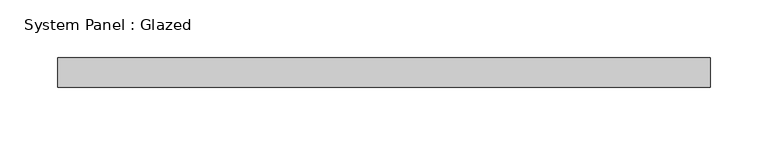
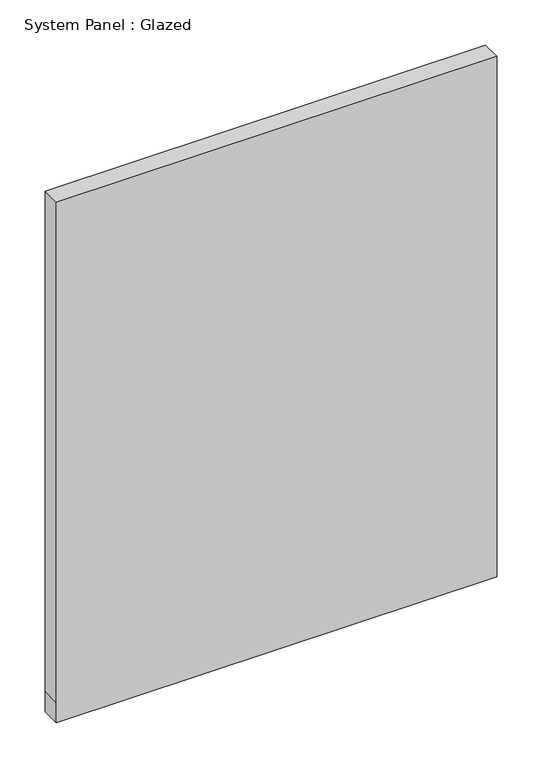
"""IFC4 building model written with IfcOpenShell, lengths in millimetres: plate geometry, System Panel : Glazed."""

from ifc_helpers import new_model, si_unit, frame, origin, place, context, project, spatial, polyline, outline, extrude, source, transform, mapped, element, save


def system_panel_glazed_b692d746(model_context):
    return source(origin(), model_context, "Body", "SweptSolid", [
        extrude(outline(polyline([(0.0, -282.575), (0.0, 282.575), (27.5166667, 282.575), (705.432512, 282.575), (705.432512, -282.575), (27.5166667, -282.575), (0.0, -282.575)])), frame((0.0, 19.05, 0.0), z_axis=(0.0, 1.0, 0.0), x_axis=(0.0, 0.0, 1.0)), (0.0, 0.0, 1.0), 25.4),
    ])


if __name__ == "__main__":
    model = new_model("IFC4")
    model_context = context("Model", 3, world=origin())
    ifc_project = project(units=[si_unit("LENGTHUNIT", "METRE", prefix="MILLI")], contexts=[model_context])
    site = spatial("IfcSite", under=ifc_project)
    building = spatial("IfcBuilding", under=site)
    placement = place(None, origin())
    system_panel_glazed_shape = system_panel_glazed_b692d746(model_context)
    element("IfcPlate", 1, ObjectType="System Panel : Glazed", at=placement, inside=building, context=model_context, shape_type="MappedRepresentation", body=[
        mapped(system_panel_glazed_shape, transform((0.0, 0.0, 0.0), x_axis=(1.0, 0.0, 0.0), y_axis=(0.0, 1.0, 0.0), z_axis=(0.0, 0.0, 1.0))),
    ])
    save(model, "model.ifc")

# Revit data of these elements
# Type "System Panel : Glazed"
#   Construction Type Id = "GSP4R"
#   Analytic Construction = "1/8 in Pilkington single glazing"
#   Visual Light Transmittance = 0.9
#   Solar Heat Gain Coefficient = 0.86
#   Heat Transfer Coefficient (U) = 1.18115 BTU/(h·ft²·°F)
#   Define Thermal Properties by = 1
# Element 1 (IfcPlate, "System Panel : Glazed")
#   Materials on its faces: "Glass"
# Materials
#   "Glass": class "Glass", colour RGB 0 128 192, transparency 0.75, Description = "Soda Lime Glass", Cost = 0
